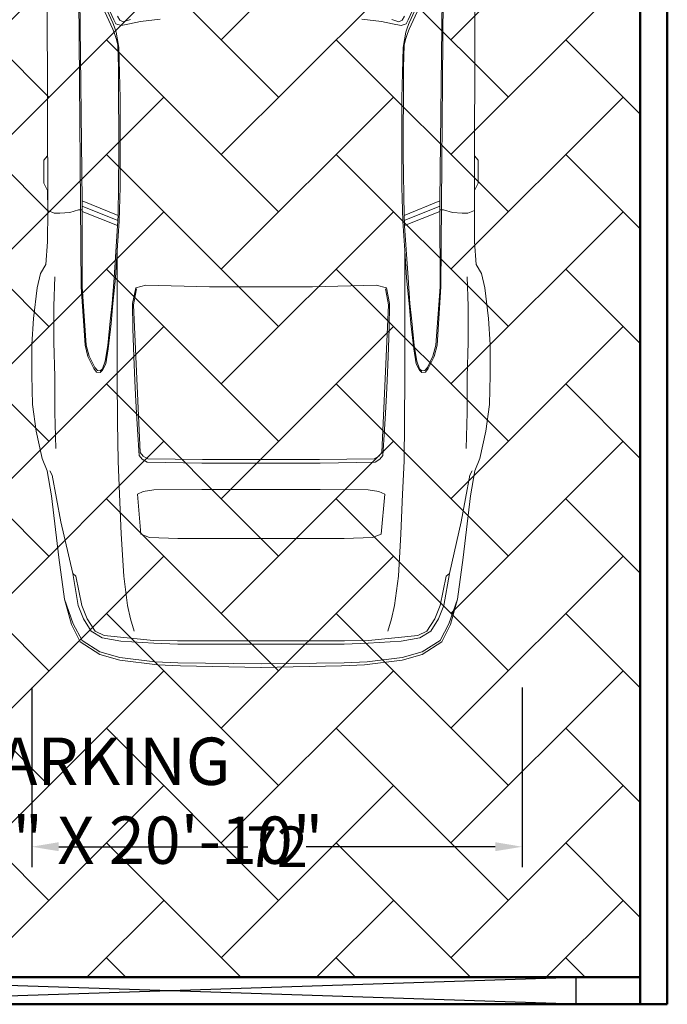
# Model space of a CAD drawing. Units: inches. Extents: x -466983 to 1020, y 324 to 318697.
# Tile 24 of 97: x 896 to 992, y 365 to 511. Entities that reach past the tile are written whole.
import ezdxf

# ---------------------------------------------------------------- set-up
doc = ezdxf.new("R2010")
doc.units = ezdxf.units.IN
doc.header["$MEASUREMENT"] = 0
for name, color, linetype, lineweight in [('A-ANNO-DIMS', 2, 'Continuous', 18), ('A-AREA-IDEN', 7, 'Continuous', 25), ('A-DOOR', 3, 'Continuous', 25), ('A-EQPM-VEHC', 8, 'Continuous', 18), ('A-FLOR-PATT', 252, 'Continuous', 13), ('A-WALL', 7, 'Continuous', 50)]:
    doc.layers.add(name, color=color, linetype=linetype, lineweight=lineweight)
doc.styles.get("Standard").update_dxf_attribs({"font": 'arial.ttf'})
doc.dimstyles.get("Standard").update_dxf_attribs({"dimtxt": 6, "dimasz": 4, "dimexe": 3, "dimexo": 3, "dimgap": 0.09, "dimtad": 0, "dimtih": 1, "dimtoh": 1, "dimdec": 1, "dimzin": 0, "dimdsep": 46, "dimlunit": 3, "dimtxsty": 'Standard', "dimcen": 0.09, "dimadec": 0, "dimazin": 0, "dimtfac": 1, "dimtdec": 1, "dimtofl": 0, "dimtmove": 0, "dimatfit": 3, "dimfxl": 1, "dimtolj": 1, "dimtzin": 0, "dimarcsym": 0})

# ---------------------------------------------------------------- blocks, each defined once
blk = doc.blocks.new('A$C7AB76BE8')
for p, q in [((2866.4, 1606.5), (2916.9, 1619)), ((2916.9, 1619), (3027.4, 1632)), ((3027.4, 1632), (3119.4, 1638)), ((3119.4, 1638), (3229.9, 1638)), ((3229.9, 1638), (3334.4, 1635)), ((3334.4, 1635), (3429.4, 1622.5)), ((3429.4, 1622.5), (3527.4, 1600.5)), ((2445.4, 1581.9), (2461.4, 1594.4)), ((2461.4, 1594.4), (2543.4, 1594.4)), ((2543.4, 1594.4), (2568.9, 1581.9)), ((2753.2, 1581.5), (2834.4, 1587.5)), ((2834.4, 1587.5), (2866.4, 1606.5)), ((3527.4, 1600.5), (3571.8, 1582.3)), ((1736.1, 1582.8), (2641.4, 1581.1)), ((2438.9, 1581.9), (2445.4, 1581.9)), ((2568.9, 1581.9), (2603.4, 1581.9)), ((2641.4, 1581.1), (2753.2, 1581.5)), ((2650.9, 1557.3), (2641.4, 1581.1)), ((2650.9, 1537.9), (2650.9, 1557.3)), ((2878, 1555.4), (2982.5, 1558.8)), ((2982.5, 1558.8), (3112, 1558.8)), ((3112, 1558.8), (3235.5, 1555.4)), ((3235.5, 1555.4), (3363.3, 1555.4)), ((3363.3, 1555.4), (3491.5, 1551.9)), ((3571.8, 1582.3), (3660.3, 1566.8)), ((3571.8, 1573.7), (3587.4, 1565.1)), ((3587.4, 1565.1), (3754, 1533.6)), ((3660.3, 1566.8), (3881.8, 1540.9)), ((2647.9, 1502.5), (2650.9, 1537.9)), ((3754, 1533.6), (3938.8, 1491.7)), ((3881.8, 1540.9), (4030.3, 1521)), ((4120.8, 1496.3), (4030.3, 1521)), ((4030.3, 1521), (4118.9, 1490.4)), ((2638.4, 1470.5), (2647.9, 1502.5)), ((3938.8, 1491.7), (4052.8, 1472.3)), ((3938.8, 1491.7), (3948.3, 1480.9)), ((3948.3, 1480.9), (4052.8, 1459.3)), ((4118.9, 1490.4), (4178.4, 1458.4)), ((4182.3, 1464.5), (4120.8, 1496.3)), ((1720.9, 1453.3), (1959.3, 1344.9)), ((2913.9, 1461.5), (1727.4, 1470.5)), ((1734.3, 1455.8), (1970.1, 1348.3)), ((2189.8, 1462.8), (1741.2, 1467.5)), ((1756.8, 1455.8), (1992.5, 1348.3)), ((2606.9, 1458), (2189.8, 1462.8)), ((2638.4, 1458), (2606.9, 1458)), ((2606.9, 1458), (2658.3, 1329.8)), ((2625.4, 1458), (2676.8, 1330.6)), ((2638.4, 1458), (2638.4, 1470.5)), ((2913.9, 1458.4), (2638.4, 1458)), ((2644, 1458), (2695, 1331.5)), ((3122.4, 1447.6), (2913.9, 1461.5)), ((3122.8, 1443.8), (2913.9, 1458.4)), ((3163, 1437.7), (3122.4, 1447.6)), ((3161.2, 1433), (3122.8, 1443.8)), ((4052.8, 1472.3), (4099.9, 1452.8)), ((4052.8, 1459.3), (4099.9, 1439.9)), ((4099.9, 1452.8), (4144.3, 1426.1)), ((4178.4, 1458.4), (4219, 1394.5)), ((4228.5, 1394.5), (4182.3, 1464.5)), ((3201.8, 1413.1), (3161.2, 1433)), ((3206.1, 1416.6), (3163, 1437.7)), ((3213.1, 1403.6), (3201.8, 1413.1)), ((3219.1, 1406.6), (3206.1, 1416.6)), ((4099.9, 1439.9), (4144.3, 1411.4)), ((4144.3, 1426.1), (4168.1, 1386.8)), ((4144.3, 1411.4), (4160.3, 1379)), ((3123.2, 1366), (3179.8, 1375.1)), ((3135.1, 1364.6), (3189, 1373.7)), ((3179.8, 1375.1), (3207, 1385)), ((3189, 1373.7), (3211.8, 1385)), ((3207, 1385), (3213.5, 1393.2)), ((3211.8, 1385), (3220.4, 1393.7)), ((3213.5, 1393.2), (3213.1, 1403.6)), ((3220.4, 1393.7), (3219.1, 1406.6)), ((4160.3, 1379), (4178.3, 1202.8)), ((4168.1, 1386.8), (4180.2, 1319.8)), ((4219, 1394.5), (4238.9, 1322.9)), ((4248.4, 1322.9), (4228.5, 1394.5)), ((1959.3, 1344.9), (1973.5, 1337.5)), ((1970.1, 1348.3), (1986, 1342.3)), ((1973.5, 1337.5), (1979.6, 1319)), ((1986, 1342.3), (2003.3, 1336.3)), ((1992.5, 1348.3), (2008.5, 1342.3)), ((2008.5, 1342.3), (2025.8, 1336.3)), ((2695.4, 1331.5), (2881.9, 1344)), ((2783.9, 1332.4), (2881.9, 1338.8)), ((2881.9, 1344), (2973.9, 1350.5)), ((2881.9, 1338.8), (2973.2, 1348.1)), ((2973.2, 1348.1), (3044.4, 1354.2)), ((2973.9, 1350.5), (3036, 1357.4)), ((3036, 1357.4), (3123.2, 1366)), ((3044.4, 1354.2), (3135.1, 1364.6)), ((1946.3, 1331.9), (1960.6, 1323.3)), ((1966.2, 1311.6), (1958.8, 1285.7)), ((1960.6, 1323.3), (1966.2, 1311.6)), ((1979.6, 1319), (1973.5, 1289.2)), ((2003.3, 1336.3), (2058.1, 1326.3)), ((2025.8, 1336.3), (2049.1, 1330.2)), ((2049.1, 1330.2), (2130.7, 1327.6)), ((2058.1, 1326.3), (2239.9, 1322)), ((2130.7, 1327.6), (2239.5, 1327.6)), ((2239.5, 1327.6), (2354.7, 1327.2)), ((2239.9, 1322), (2438.9, 1322)), ((2354.7, 1327.2), (2439.4, 1326.3)), ((2438.9, 1322), (2558.1, 1322)), ((2439.4, 1326.3), (2658.3, 1329.8)), ((2558.1, 1322), (2679, 1325.2)), ((2658.3, 1329.8), (2695.4, 1331.5)), ((2679, 1325.2), (2783.9, 1332.4)), ((2783.9, 1332.4), (3236.4, 1333.2)), ((3236.4, 1333.2), (3397.8, 1331.5)), ((3397.8, 1331.5), (3536.9, 1329.8)), ((3536.9, 1329.8), (3655.2, 1324.6)), ((3655.2, 1324.6), (3797.2, 1318.1)), ((3797.2, 1318.1), (3948.3, 1309.5)), ((3948.3, 1309.5), (4052.8, 1296.1)), ((4180.2, 1319.8), (4187.9, 1201.5)), ((4238.9, 1322.9), (4254.4, 1198.1)), ((4264.8, 1188.6), (4248.4, 1322.9)), ((1973.5, 1289.2), (1965.7, 1249.5)), ((2916.9, 1266.7), (2973.4, 1278.4)), ((2977.8, 1274.9), (2921.2, 1263.3)), ((2973.4, 1278.4), (3064.1, 1276.7)), ((3505.8, 1250.8), (2977.8, 1274.9)), ((3064.1, 1276.7), (3162.5, 1273.7)), ((3162.5, 1273.7), (3249.8, 1269.3)), ((3249.8, 1269.3), (3300.3, 1267.6)), ((3300.3, 1267.6), (3365.5, 1263.7)), ((4052.8, 1296.1), (4099.9, 1285.3)), ((4099.9, 1285.3), (4144.3, 1272.4)), ((1965.7, 1249.5), (1957.5, 1179.5)), ((2907.4, 1230.5), (2916.9, 1266.7)), ((3365.5, 1263.7), (3423.3, 1260.3)), ((3423.3, 1260.3), (3516.6, 1254.2)), ((3519.2, 1240), (3505.8, 1250.8)), ((3516.6, 1254.2), (3530, 1243)), ((3529.1, 1222.7), (3519.2, 1240)), ((3530, 1243), (3540.3, 1226.2)), ((3645.2, 1240.4), (3638.8, 1202)), ((3654.7, 1260.7), (3645.2, 1240.4)), ((3797.6, 1248.2), (3654.7, 1260.7)), ((3809.7, 1217.5), (3797.6, 1248.2)), ((2913.4, 1002.5), (2907.4, 1230.5)), ((3531.2, 1027.6), (3529.1, 1222.7)), ((3540.3, 1226.2), (3543.8, 1030.6)), ((3638.8, 1202), (3637.9, 1030.6)), ((3813.2, 1116.1), (3809.7, 1217.5)), ((4178.3, 1202.8), (4179.5, 1117.3)), ((4187.9, 1201.5), (4191, 1116.5)), ((4254.4, 1198.1), (4257.9, 1115.6)), ((4268.2, 1106.1), (4264.8, 1188.6)), ((3813.2, 819), (3813.2, 1116.1)), ((4179.5, 520.7), (4179.5, 1117.3)), ((4191, 1116.5), (4191, 521.5)), ((4257.9, 1115.6), (4261.3, 819)), ((4273.9, 819.5), (4268.2, 1106.1)), ((3531.2, 818.6), (3531.2, 1027.6)), ((3543.8, 1030.6), (3543.8, 819)), ((3637.9, 1030.6), (3637.9, 819)), ((2913.9, 818.6), (2913.4, 1002.5)), ((2913.9, 819.5), (2913.4, 635.5)), ((3531.2, 819.5), (3531.2, 610.5)), ((3543.8, 607.5), (3543.8, 819)), ((3637.9, 607.5), (3637.9, 819)), ((3813.2, 819), (3813.2, 522)), ((4257.9, 522.4), (4261.3, 819)), ((4273.9, 818.6), (4268.2, 531.9)), ((2913.4, 635.5), (2907.4, 407.6)), ((3531.2, 610.5), (3529.1, 415.3)), ((3540.3, 411.9), (3543.8, 607.5)), ((3638.8, 436.1), (3637.9, 607.5)), ((4268.2, 531.9), (4264.8, 449.4)), ((3813.2, 522), (3809.7, 420.5)), ((4178.3, 435.3), (4179.5, 520.7)), ((4187.9, 436.5), (4191, 521.5)), ((4254.4, 439.9), (4257.9, 522.4)), ((1965.7, 388.6), (1957.5, 458.5)), ((3645.2, 397.6), (3638.8, 436.1)), ((4160.3, 259), (4178.3, 435.3)), ((4180.2, 318.2), (4187.9, 436.5)), ((4238.9, 315.2), (4254.4, 439.9)), ((4264.8, 449.4), (4248.4, 315.2)), ((1973.5, 348.9), (1965.7, 388.6)), ((2907.4, 407.6), (2916.9, 371.3)), ((3505.8, 387.3), (2977.8, 363.1)), ((3519.2, 398.1), (3505.8, 387.3)), ((3516.6, 383.8), (3530, 395)), ((3529.1, 415.3), (3519.2, 398.1)), ((3530, 395), (3540.3, 411.9)), ((3654.7, 377.3), (3645.2, 397.6)), ((3797.6, 389.9), (3654.7, 377.3)), ((3809.7, 420.5), (3797.6, 389.9)), ((1966.2, 326.4), (1958.8, 352.3)), ((2916.9, 371.3), (2973.4, 359.6)), ((2977.8, 363.1), (2921.2, 374.8)), ((2973.4, 359.6), (3064.1, 361.4)), ((3064.1, 361.4), (3162.5, 364.4)), ((3162.5, 364.4), (3249.8, 368.7)), ((3249.8, 368.7), (3300.3, 370.4)), ((3300.3, 370.4), (3365.5, 374.3)), ((3365.5, 374.3), (3423.3, 377.8)), ((3423.3, 377.8), (3516.6, 383.8)), ((4052.8, 341.9), (4099.9, 352.7)), ((4099.9, 352.7), (4144.3, 365.7)), ((1960.6, 314.7), (1966.2, 326.4)), ((1979.6, 319.1), (1973.5, 348.9)), ((1973.5, 300.5), (1979.6, 319.1)), ((3655.2, 313.4), (3797.2, 319.9)), ((3797.2, 319.9), (3948.3, 328.6)), ((3948.3, 328.6), (4052.8, 341.9)), ((4168.1, 251.3), (4180.2, 318.2)), ((1720.9, 184.8), (1959.3, 293.2)), ((1734.3, 182.2), (1970.1, 289.7)), ((1756.8, 182.2), (1992.5, 289.7)), ((1946.3, 306.1), (1960.6, 314.7)), ((1959.3, 293.2), (1973.5, 300.5)), ((1970.1, 289.7), (1986, 295.7)), ((1986, 295.7), (2003.3, 301.8)), ((1992.5, 289.7), (2008.5, 295.7)), ((2003.3, 301.8), (2058.1, 311.7)), ((2008.5, 295.7), (2025.8, 301.8)), ((2025.8, 301.8), (2049.1, 307.8)), ((2049.1, 307.8), (2130.7, 310.4)), ((2058.1, 311.7), (2239.9, 316)), ((2130.7, 310.4), (2239.5, 310.4)), ((2239.5, 310.4), (2354.7, 310.9)), ((2239.9, 316), (2438.9, 316)), ((2354.7, 310.9), (2439.4, 311.7)), ((2438.9, 316), (2558.1, 316)), ((2439.4, 311.7), (2658.3, 308.3)), ((2558.1, 316), (2679, 312.8)), ((2606.9, 180), (2658.3, 308.3)), ((2625.4, 180), (2676.8, 307.4)), ((2644, 180), (2695, 306.5)), ((2658.3, 308.3), (2695.4, 306.5)), ((2679, 312.8), (2783.9, 305.7)), ((2695.4, 306.5), (2881.9, 294)), ((2783.9, 305.7), (3236.4, 304.8)), ((2783.9, 305.7), (2881.9, 299.2)), ((2881.9, 299.2), (2973.2, 290)), ((2881.9, 294), (2973.9, 287.5)), ((2973.2, 290), (3044.4, 283.9)), ((2973.9, 287.5), (3036, 280.6)), ((3044.4, 283.9), (3135.1, 273.4)), ((3236.4, 304.8), (3397.8, 306.5)), ((3397.8, 306.5), (3536.9, 308.3)), ((3536.9, 308.3), (3655.2, 313.4)), ((4219, 243.5), (4238.9, 315.2)), ((4248.4, 315.2), (4228.5, 243.5)), ((3036, 280.6), (3123.2, 272)), ((3123.2, 272), (3179.8, 262.9)), ((3135.1, 273.4), (3189, 264.3)), ((3179.8, 262.9), (3207, 253)), ((3189, 264.3), (3211.8, 253)), ((3207, 253), (3213.5, 244.8)), ((3211.8, 253), (3220.4, 244.4)), ((4144.3, 226.7), (4160.3, 259)), ((4144.3, 212), (4168.1, 251.3)), ((3201.8, 224.9), (3161.2, 205.1)), ((3206.1, 221.5), (3163, 200.3)), ((3213.1, 234.4), (3201.8, 224.9)), ((3219.1, 231.4), (3206.1, 221.5)), ((3213.5, 244.8), (3213.1, 234.4)), ((3220.4, 244.4), (3219.1, 231.4)), ((4099.9, 198.2), (4144.3, 226.7)), ((4099.9, 185.2), (4144.3, 212)), ((4178.4, 179.6), (4219, 243.5)), ((4228.5, 243.5), (4182.3, 173.6)), ((2913.9, 176.6), (1727.4, 167.5)), ((2606.9, 180), (2189.8, 175.3)), ((2638.4, 180), (2606.9, 180)), ((2638.4, 180), (2638.4, 167.5)), ((2913.9, 179.6), (2638.4, 180)), ((3122.8, 194.3), (2913.9, 179.6)), ((3122.4, 190.4), (2913.9, 176.6)), ((3163, 200.3), (3122.4, 190.4)), ((3161.2, 205.1), (3122.8, 194.3)), ((3948.3, 157.2), (4052.8, 178.7)), ((4052.8, 178.7), (4099.9, 198.2)), ((4052.8, 165.8), (4099.9, 185.2)), ((4118.9, 147.7), (4178.4, 179.6)), ((2189.8, 175.3), (1741.2, 170.5)), ((2638.4, 167.5), (2647.9, 135.6)), ((3754, 104.5), (3938.8, 146.4)), ((3938.8, 146.4), (4052.8, 165.8)), ((3938.8, 146.4), (3948.3, 157.2)), ((4030.3, 117), (4118.9, 147.7)), ((4120.8, 141.8), (4030.3, 117)), ((4182.3, 173.6), (4120.8, 141.8)), ((2647.9, 135.6), (2650.9, 100.2)), ((3881.8, 97.1), (4030.3, 117)), ((2650.9, 80.7), (2641.4, 57)), ((2650.9, 100.2), (2650.9, 80.7)), ((2878, 82.7), (2982.5, 79.2)), ((2982.5, 79.2), (3112, 79.2)), ((3112, 79.2), (3235.5, 82.7)), ((3235.5, 82.7), (3363.3, 82.7)), ((3363.3, 82.7), (3491.5, 86.1)), ((3571.8, 64.3), (3587.4, 73)), ((3571.8, 55.7), (3660.3, 71.2)), ((3587.4, 73), (3754, 104.5)), ((3660.3, 71.2), (3881.8, 97.1)), ((1736.1, 55.3), (2641.4, 57)), ((2438.9, 56.1), (2445.4, 56.1)), ((2445.4, 56.1), (2461.4, 43.6)), ((2461.4, 43.6), (2543.4, 43.6)), ((2543.4, 43.6), (2568.9, 56.1)), ((2568.9, 56.1), (2603.4, 56.1)), ((2641.4, 57), (2753.2, 56.6)), ((2753.2, 56.6), (2834.4, 50.5)), ((2834.4, 50.5), (2866.4, 31.5)), ((3429.4, 15.5), (3527.4, 37.6)), ((3527.4, 37.6), (3571.8, 55.7)), ((2866.4, 31.5), (2916.9, 19)), ((2916.9, 19), (3027.4, 6)), ((3027.4, 6), (3119.4, 0)), ((3119.4, 0), (3229.9, 0)), ((3229.9, 0), (3334.4, 3)), ((3334.4, 3), (3429.4, 15.5))]:
    blk.add_line(p, q)
blk = doc.blocks.new('*D95')
at = {"layer": 'A-ANNO-DIMS', "color": 0, "lineweight": -2, "transparency": 16777216}
for p, q in [((894.88, 591.6), (868.36, 591.6)), ((871.36, 587.6), (871.36, 506.38)), ((871.36, 418.77), (871.36, 499.99)), ((894.88, 414.77), (868.36, 414.77))]:
    blk.add_line(p, q, dxfattribs=at)
at = {"layer": 'A-ANNO-DIMS', "color": 0, "transparency": 16777216}
for points in [[(870.69, 587.6), (872.03, 587.6), (871.36, 591.6)], [(870.69, 418.77), (872.03, 418.77), (871.36, 414.77)]]:
    blk.add_solid(points, dxfattribs=at)
at = {"layer": 'Defpoints', "color": 0, "transparency": 16777216}
for p in [(897.88, 591.6), (871.36, 414.77), (897.88, 414.77)]:
    blk.add_point(p, dxfattribs=at)
at = {"layer": 'A-ANNO-DIMS', "color": 0, "transparency": 16777216, "insert": (871.36, 503.18), "char_height": 6, "attachment_point": 5}
blk.add_mtext('\\A1;CAR 177', dxfattribs=at)
blk = doc.blocks.new('*D96')
at = {"layer": 'A-ANNO-DIMS', "color": 0, "lineweight": -2, "transparency": 16777216}
for p, q in [((897.88, 411.77), (897.88, 385.24)), ((970.37, 411.77), (970.37, 385.24)), ((901.88, 388.24), (929.8, 388.24)), ((966.37, 388.24), (938.46, 388.24))]:
    blk.add_line(p, q, dxfattribs=at)
at = {"layer": 'A-ANNO-DIMS', "color": 0, "transparency": 16777216}
for points in [[(901.88, 388.91), (901.88, 387.58), (897.88, 388.24)], [(966.37, 388.91), (966.37, 387.58), (970.37, 388.24)]]:
    blk.add_solid(points, dxfattribs=at)
at = {"layer": 'Defpoints', "color": 0, "transparency": 16777216}
for p in [(897.88, 414.77), (970.37, 414.77), (970.37, 388.24)]:
    blk.add_point(p, dxfattribs=at)
at = {"layer": 'A-ANNO-DIMS', "color": 0, "transparency": 16777216, "insert": (934.13, 388.24), "char_height": 6, "attachment_point": 5}
blk.add_mtext('\\A1;72', dxfattribs=at)

msp = doc.modelspace()

# ---------------------------------------------------------------- hatches: boundary and pattern name
at = {"layer": 'A-FLOR-PATT', "transparency": 33554572}
h = msp.add_hatch(dxfattribs=at)
h.set_pattern_fill('AR-HBONE', color=256, scale=3)
h.set_pattern_definition([(45, (-1212.414, -290.035), (0, 16.97056), [36, -12]), (135, (-1203.928, -281.55), (1e-15, 16.97056), [36, -12])])
h.paths.add_polyline_path([(987.81, 618.94), (813.81, 618.94), (813.81, 368.94), (987.81, 368.94)])

# ---------------------------------------------------------------- linework, layer by layer
at = {"layer": 'A-DOOR'}
for p, q in [((856.65, 364.94), (978.34, 368.94)), ((978.34, 364.94), (856.65, 368.94)), ((978.34, 364.94), (978.34, 368.94))]:
    msp.add_line(p, q, dxfattribs=at)
at = {"layer": 'A-WALL'}
for p, q in [((991.81, 1084.94), (991.81, 364.94)), ((987.81, 618.94), (987.81, 364.94)), ((987.81, 368.94), (395.81, 368.94)), ((991.81, 364.94), (391.81, 364.94))]:
    msp.add_line(p, q, dxfattribs=at)

# ---------------------------------------------------------------- block references
at = {"layer": 'A-EQPM-VEHC', "xscale": 0.0413745961844617, "yscale": 0.0413745961844617, "zscale": 0.0413745961844617, "rotation": 270}
msp.add_blockref('A$C7AB76BE8', (897.88, 591.6), dxfattribs=at)

# ---------------------------------------------------------------- texts
at = {"layer": 'A-AREA-IDEN', "insert": (792.28, 404.38), "char_height": 7, "attachment_point": 1}
msp.add_mtext_dynamic_manual_height_columns('\\pxqc;{\\fArial|b1|i0|c0|p34;PARKING\\P14\'-6" X 20\'-10"}', width=229.5583, gutter_width=1, heights=[0], dxfattribs=at)

# ---------------------------------------------------------------- dimensions: what is measured, and where the dimension line sits
at = {"layer": 'A-ANNO-DIMS'}
dim = msp.add_linear_dim(base=(871.36, 414.77), p1=(897.88, 591.6), p2=(897.88, 414.77), angle=270, text='CAR <>', dimstyle='Standard', override={"dimdec": 0, "dimlfac": 1, "dimrnd": 0, "dimzin": 0, "dimdsep": 46, "dimlunit": 2}, dxfattribs=at)
dim.commit()
dim.dimension.update_dxf_attribs({"geometry": '*D95', "text_midpoint": (871.36, 503.18)})
dim = msp.add_linear_dim(base=(970.37, 388.24), p1=(897.88, 414.77), p2=(970.37, 414.77), dimstyle='Standard', override={"dimdec": 0, "dimlfac": 1, "dimrnd": 0, "dimzin": 0, "dimdsep": 46, "dimlunit": 2}, dxfattribs=at)
dim.commit()
dim.dimension.update_dxf_attribs({"geometry": '*D96', "text_midpoint": (934.13, 388.24)})

doc.saveas('drawing.dxf')
